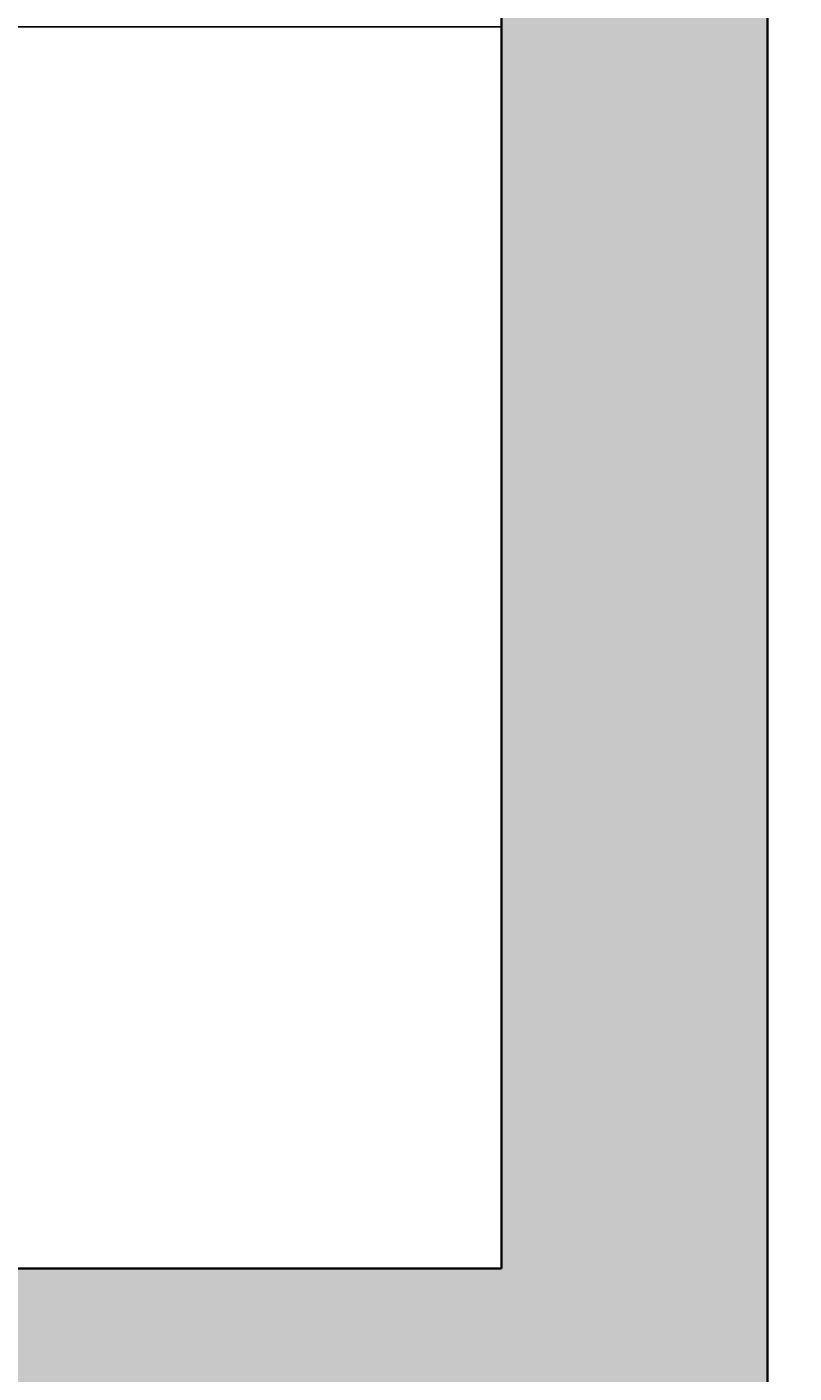
# Model space of a CAD drawing. Units: inches. Extents: x 1998 to 2588, y 1139 to 1977.
# Tile 115 of 134: x 2524 to 2550, y 1477 to 1523. Entities that reach past the tile are written whole.
import ezdxf

# ---------------------------------------------------------------- set-up
doc = ezdxf.new("R2010")
doc.units = ezdxf.units.IN
for name, color, linetype, lineweight in [('A-ANNO-DIMS', 2, 'Continuous', 18), ('A-FLOR-STRS', 7, 'Continuous', 25), ('A-WALL-PATT', 252, 'Continuous', 13), ('WALL', 200, 'Continuous', 35)]:
    doc.layers.add(name, color=color, linetype=linetype, lineweight=lineweight)
doc.styles.get("Standard").update_dxf_attribs({"font": 'arial.ttf'})
doc.dimstyles.get("Standard").update_dxf_attribs({"dimtxt": 0.18, "dimasz": 0.18, "dimexe": 0.18, "dimexo": 0.0625, "dimgap": 0.09, "dimtad": 0, "dimtih": 1, "dimtoh": 1, "dimdec": 4, "dimzin": 0, "dimdsep": 46, "dimtxsty": 'Standard', "dimcen": 0.09, "dimadec": 0, "dimazin": 0, "dimtfac": 1, "dimtdec": 4, "dimtofl": 0, "dimtmove": 0, "dimatfit": 3, "dimfxl": 1, "dimtolj": 1, "dimtzin": 0, "dimarcsym": 0})

# ---------------------------------------------------------------- blocks, each defined once
blk = doc.blocks.new('*D24')
at = {"layer": 'A-ANNO-DIMS', "color": 0, "lineweight": -2, "transparency": 16777216}
for p, q in [((2398.535, 1911.232), (2588.309, 1911.232)), ((2588.129, 1911.052), (2588.129, 1570.164)), ((2588.129, 1228.912), (2588.129, 1569.8)), ((2527.535, 1228.732), (2588.309, 1228.732))]:
    blk.add_line(p, q, dxfattribs=at)
at = {"layer": 'A-ANNO-DIMS', "color": 0, "transparency": 16777216}
for points in [[(2588.099, 1911.052), (2588.159, 1911.052), (2588.129, 1911.232)], [(2588.099, 1228.912), (2588.159, 1228.912), (2588.129, 1228.732)]]:
    blk.add_solid(points, dxfattribs=at)
at = {"layer": 'Defpoints', "color": 0, "transparency": 16777216}
for p in [(2398.473, 1911.232), (2588.129, 1911.232), (2527.473, 1228.732)]:
    blk.add_point(p, dxfattribs=at)
at = {"layer": 'A-ANNO-DIMS', "color": 0, "transparency": 16777216, "insert": (2588.129, 1569.982), "char_height": 0.18, "attachment_point": 5}
blk.add_mtext('\\A1;682.5', dxfattribs=at)

msp = doc.modelspace()

# ---------------------------------------------------------------- hatches: boundary and pattern name
at = {"layer": 'A-WALL-PATT'}
h = msp.add_hatch(color=256, dxfattribs=at)
h.dxf.hatch_style = 1
h.paths.add_polyline_path([(2527.4729, 1362.2324), (2510.9729, 1362.2324), (2510.9729, 1357.7324), (2518.4729, 1357.7324), (2518.4729, 1237.7324), (2503.1458, 1237.7324), (2503.1458, 1228.7324), (2527.4729, 1228.7324)])
h.paths.add_polyline_path([(2490.5682, 1362.2324), (2398.4729, 1362.2324), (2398.4729, 1357.7324), (2490.5682, 1357.7324)])
h.paths.add_polyline_path([(2224.9729, 1264.7324), (2222.9729, 1264.7324), (2222.9729, 1232.4125), (2341.4729, 1232.4125), (2341.4729, 1234.4125), (2224.9729, 1234.4125)])
h.paths.add_polyline_path([(2334.5332, 1273.7324), (2264.7638, 1273.7324), (2264.7638, 1269.5611, -0.043659), (2264.3413, 1264.7324), (2334.5332, 1264.7324)])
h.paths.add_polyline_path([(2236.9551, 1273.7324), (2234.4125, 1273.7324), (2234.4125, 1264.7324), (2236.9551, 1264.7324), (2236.9551, 1269.5611)])
h.paths.add_polyline_path([(2222.9729, 1293.2324), (2096.9729, 1293.2324), (2096.9729, 1345.0966), (2087.9729, 1345.0966), (2087.9729, 1284.2324), (2222.9729, 1284.2324), (2222.9729, 1285.137)])
h.paths.add_polyline_path([(2096.9729, 1458.7927), (2087.9729, 1458.7927), (2087.9729, 1417.7324), (2087.9729, 1413.2324), (2096.9729, 1413.2324), (2096.9729, 1417.7324)])
h.paths.add_polyline_path([(2096.9729, 1413.2324), (2087.9729, 1413.2324), (2087.9729, 1365.5012), (2096.9729, 1365.5012), (2096.9729, 1369.3358)])
h.paths.add_polyline_path([(2186.2943, 1417.7324), (2138.6074, 1417.7324), (2096.9729, 1417.7324), (2096.9729, 1413.2324), (2138.6074, 1413.2324), (2186.2943, 1413.2324)])
h.paths.add_polyline_path([(2181.4729, 1465.7324), (2176.9729, 1465.7324), (2176.9729, 1451.6434), (2181.4729, 1451.6434)])
h.paths.add_polyline_path([(2181.4729, 1422.1664), (2176.9729, 1422.1664), (2176.9729, 1417.7324), (2181.4729, 1417.7324)])
h.paths.add_polyline_path([(2063.9729, 1465.7324), (2087.9729, 1465.7324), (2087.9729, 1470.2324), (2059.4729, 1470.2324), (2059.4729, 1413.2324), (2087.9729, 1413.2324), (2087.9729, 1417.7324), (2063.9729, 1417.7324)])
h.paths.add_polyline_path([(2181.4729, 1755.2324), (2176.9729, 1755.2324), (2176.9729, 1748.6798), (2177.0513, 1748.6798), (2181.4729, 1748.6798)])
h.paths.add_polyline_path([(2227.4729, 1707.2324), (2220.4647, 1707.2324), (2220.4647, 1702.7324), (2222.9729, 1702.7324), (2222.9729, 1604.637), (2227.4729, 1604.637)])
h.paths.add_polyline_path([(2114.9729, 1702.7324), (2105.9729, 1702.7324), (2105.9729, 1628.4781, -0.0318759), (2110.1012, 1628.7416), (2114.9729, 1628.7416)])
h.paths.add_polyline_path([(2345.9729, 1739.3278), (2341.4729, 1739.3278), (2341.4729, 1647.5211), (2345.9729, 1647.5211)])
h.paths.add_polyline_path([(2350.6273, 1641.2324), (2345.9729, 1641.2324), (2345.9729, 1636.7324), (2350.6273, 1636.7324), (2350.6273, 1639.8729)])
h.paths.add_polyline_path([(2501.9729, 1641.2324), (2407.9729, 1641.2324), (2392.5005, 1641.2324), (2392.5005, 1639.8729), (2392.5005, 1636.7324), (2501.9729, 1636.7324)])
h.paths.add_polyline_path([(2510.9729, 1755.2324), (2501.9729, 1755.2324), (2501.9729, 1641.2324), (2510.9729, 1641.2324)])
h.paths.add_polyline_path([(2549.1786, 1641.2324), (2522.3775, 1641.2324), (2522.3775, 1636.7324), (2540.1786, 1636.7324), (2540.1786, 1480.7324), (2522.3775, 1480.7324), (2522.3775, 1476.2324), (2549.1786, 1476.2324)])
h.paths.add_polyline_path([(2498.1786, 1594.7324), (2407.9729, 1594.7324), (2407.9729, 1585.7324), (2416.9729, 1585.7324), (2489.1786, 1585.7324), (2489.1786, 1531.7324), (2416.9729, 1531.7324), (2407.9729, 1531.7324), (2407.9729, 1522.7324), (2498.1786, 1522.7324)])
h.paths.add_polyline_path([(2351.6437, 1480.7324), (2345.9729, 1480.7324), (2345.9729, 1476.2324), (2351.6437, 1476.2324), (2351.6437, 1477.5919)])
h.paths.add_polyline_path([(2501.9729, 1480.7324), (2498.1786, 1480.7324), (2407.9729, 1480.7324), (2393.5168, 1480.7324), (2393.5168, 1477.5919), (2393.5168, 1476.2324), (2501.9729, 1476.2324)])

# ---------------------------------------------------------------- linework, layer by layer
at = {"layer": 'A-FLOR-STRS'}
for p, q in [((2540.1786, 1522.7324), (2407.9729, 1522.7324)), ((2540.1786, 1480.7324), (2540.1786, 1522.7324)), ((2540.1786, 1480.7324), (2498.1786, 1480.7324))]:
    msp.add_line(p, q, dxfattribs=at)
at = {"layer": 'WALL'}
for p, q in [((2549.1786, 1641.2324), (2549.1786, 1476.2324)), ((2540.1786, 1636.7324), (2540.1786, 1480.7324)), ((2540.1786, 1480.7324), (2407.9729, 1480.7324))]:
    msp.add_line(p, q, dxfattribs=at)

# ---------------------------------------------------------------- dimensions: what is measured, and where the dimension line sits
at = {"layer": 'A-ANNO-DIMS'}
dim = msp.add_linear_dim(base=(2588.1286, 1911.2324), p1=(2527.4729, 1228.7324), p2=(2398.4729, 1911.2324), angle=90, dimstyle='Standard', override={"dimdec": 1, "dimlfac": 1, "dimrnd": 0, "dimzin": 0, "dimdsep": 46, "dimlunit": 2}, dxfattribs=at)
dim.commit()
dim.dimension.update_dxf_attribs({"geometry": '*D24', "text_midpoint": (2588.1286, 1569.9824)})

doc.saveas('drawing.dxf')
